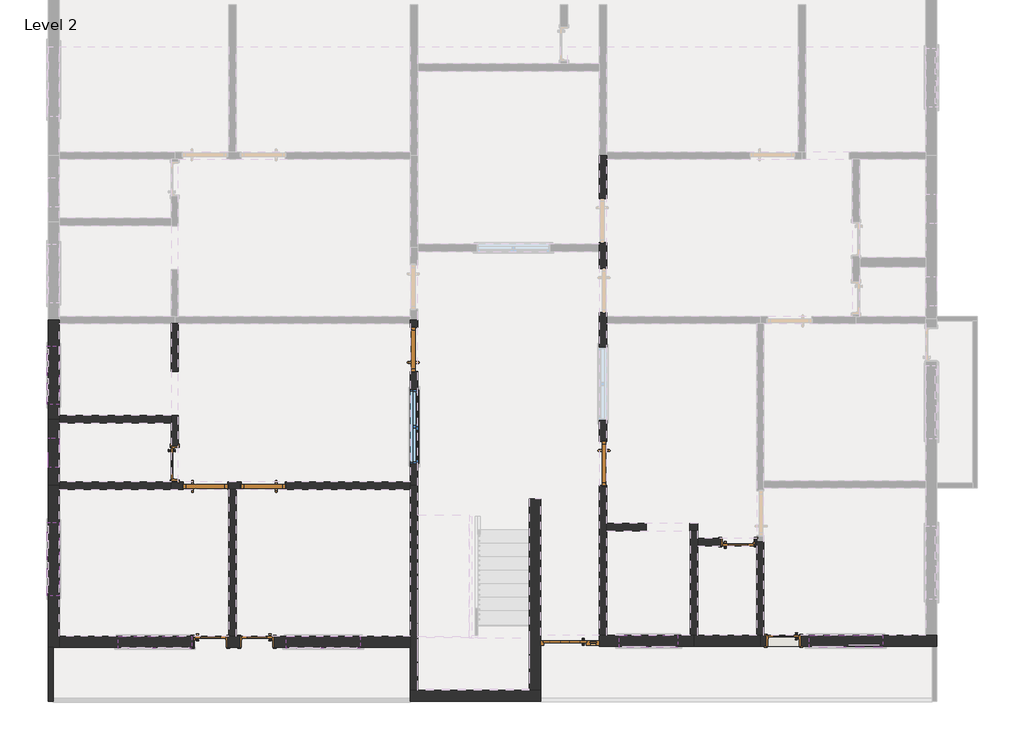
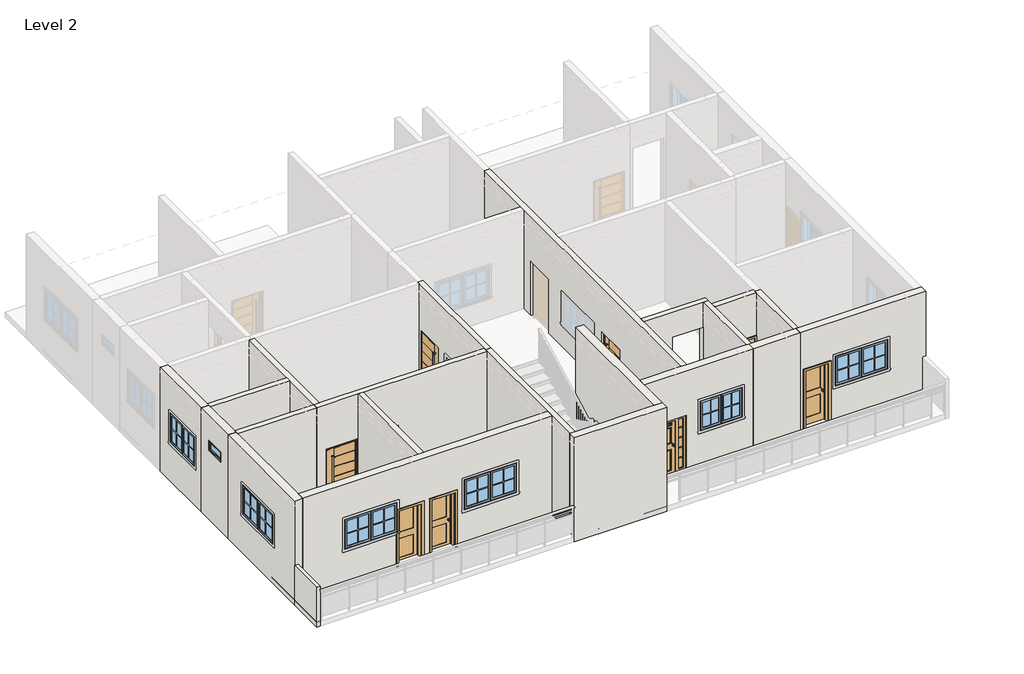
# One storey, part 1 of 5: 22 walls, 10 doors, 8 windows.
# Revit data of these elements (continued)
# Element 22 (IfcWall, "Generic - 6\"") (continued)
#   Unconnected Height = 10' - 6"
#   wall height = 10' - 6"
#   Phase Created = New Construction
#   Base Constraint = Level 2
#   Materials on its faces: "Default Wall", "BRW3", "LVW1"
# Element 23 (IfcWall, "Generic - 6\"")
#   Top Offset = 0' - 0"
#   Base Offset = 0' - 0"
#   Unconnected Height = 10' - 6"
#   wall height = 10' - 6"
#   Phase Created = New Construction
#   Base Constraint = Level 2
#   Materials on its faces: "Default Wall", "BW1", "BRW4"
# Elements 24, 27 (IfcWall, "Generic - 9\"")
#   Top Offset = 0' - 0"
#   Base Offset = 0' - 0"
#   Unconnected Height = 10' - 6"
#   wall height = 10' - 6"
#   Phase Created = New Construction
#   Base Constraint = Level 2
#   Materials on its faces: "Default Wall", "OW1", "BRW4"
# Element 25 (IfcWall, "Generic - 9\"")
#   Top Offset = 0' - 0"
#   Base Offset = 0' - 0"
#   Unconnected Height = 10' - 6"
#   wall height = 10' - 6"
#   Phase Created = New Construction
#   Base Constraint = Level 2
#   Materials on its faces: "OW1", "Default Wall", "LVW2"
# Element 26 (IfcWall, "Generic - 9\"")
#   Top Offset = 0' - 0"
#   Base Offset = 0' - 0"
#   Unconnected Height = 10' - 6"
#   wall height = 10' - 6"
#   Phase Created = New Construction
#   Base Constraint = Level 2
#   Materials on its faces: "Default Wall", "OW1"
# Element 28 (IfcWall, "Generic - 9\"")
#   Top Offset = 0' - 0"
#   Base Offset = 0' - 0"
#   Unconnected Height = 10' - 6"
#   wall height = 10' - 6"
#   Phase Created = New Construction
#   Base Constraint = Level 2
#   Materials on its faces: "Default Wall", "BW1", "OW1"
# Element 29 (IfcWall, "Generic - 9\"")
#   Top Offset = 0' - 0"
#   Base Offset = 0' - 0"
#   Unconnected Height = 10' - 6"
#   wall height = 10' - 6"
#   Phase Created = New Construction
#   Base Constraint = Level 2
#   Materials on its faces: "Default Wall", "LVW2", "OW1"
# Element 30 (IfcWall, "Generic - 9\"")
#   Top Offset = 0' - 0"
#   Base Offset = 0' - 0"
#   Unconnected Height = 10' - 6"
#   wall height = 10' - 6"
#   Phase Created = New Construction
#   Base Constraint = Level 2
#   Materials on its faces: "Default Wall", "OW1", "KW2"
# Element 31 (IfcWall, "Generic - 9\"")
#   Top Offset = 0' - 0"
#   Base Offset = 0' - 0"
#   Unconnected Height = 10' - 6"
#   wall height = 10' - 6"
#   Phase Created = New Construction
#   Base Constraint = Level 2
#   Materials on its faces: "Default Wall", "OW1", "BW1"
# Element 32 (IfcWall, "Generic - 9\"")
#   Top Offset = 0' - 0"
#   Base Offset = 0' - 0"
#   Unconnected Height = 10' - 6"
#   wall height = 10' - 6"
#   Phase Created = New Construction
#   Base Constraint = Level 2
#   Materials on its faces: "Default Wall", "OW1", "BRW3"
# Element 33 (IfcWindow, "Fixed : 2'")
#   Mark = "42"
#   Phase Created = New Construction
#   Materials on its faces: "Sash", "Glass"
# Element 34 (IfcWindow, "M_Window-Awning-Double-Horizontal : 4'")
#   Mark = "34"
#   Window Inset = 0' - 0"
#   Interior Wall Closure = 0' - 2.15551"
#   Frame Extension = 0' - 0 1/4"
#   Exterior Wall Closure = 0' - 1 1/4"
#   Interior Trim Visibility = yes
#   Exterior Trim Visibility = yes
#   Phase Created = New Construction
#   Materials on its faces: "Wood - Stained", "Glass", "Clad - White"
# Element 35 (IfcWindow, "M_Window-Awning-Double-Horizontal : 4'")
#   Mark = "35"
#   Window Inset = 0' - 0"
#   Interior Wall Closure = 0' - 2.15551"
#   Frame Extension = 0' - 0 1/4"
#   Exterior Wall Closure = 0' - 1 1/4"
#   Interior Trim Visibility = yes
#   Exterior Trim Visibility = yes
#   Phase Created = New Construction
#   Materials on its faces: "Wood - Stained", "Glass", "Clad - White"
# Element 36 (IfcWindow, "M_Window-Awning-Double-Horizontal : 5'")
#   Mark = "25"
#   Window Inset = 0' - 0"
#   Interior Wall Closure = 0' - 2 5/32"
#   Frame Extension = 0' - 0 1/4"
#   Exterior Wall Closure = 0' - 1 1/4"
#   Interior Trim Visibility = yes
#   Exterior Trim Visibility = yes
#   Phase Created = New Construction
#   Materials on its faces: "Wood - Stained", "Glass", "Clad - White"
# Element 37 (IfcWindow, "M_Window-Awning-Double-Horizontal : 5'")
#   Mark = "26"
#   Window Inset = 0' - 0"
#   Interior Wall Closure = 0' - 2 5/32"
#   Frame Extension = 0' - 0 1/4"
#   Exterior Wall Closure = 0' - 1 1/4"
#   Interior Trim Visibility = yes
#   Exterior Trim Visibility = yes
#   Phase Created = New Construction
#   Materials on its faces: "Wood - Stained", "Glass", "Clad - White"
# Element 38 (IfcWindow, "M_Window-Awning-Double-Horizontal : 5'")
#   Mark = "27"
#   Window Inset = 0' - 0"
#   Interior Wall Closure = 0' - 2 5/32"
#   Frame Extension = 0' - 0 1/4"
#   Exterior Wall Closure = 0' - 1 1/4"
#   Interior Trim Visibility = yes
#   Exterior Trim Visibility = yes
#   Phase Created = New Construction
#   Materials on its faces: "Wood - Stained", "Glass", "Clad - White"
# Element 39 (IfcWindow, "M_Window-Awning-Double-Horizontal : 5'")
#   Mark = "28"
#   Window Inset = 0' - 0"
#   Interior Wall Closure = 0' - 2 5/32"
#   Frame Extension = 0' - 0 1/4"
#   Exterior Wall Closure = 0' - 1 1/4"
#   Interior Trim Visibility = yes
#   Exterior Trim Visibility = yes
#   Phase Created = New Construction
#   Materials on its faces: "Wood - Stained", "Glass", "Clad - White"
# Element 40 (IfcWindow, "M_Window-Awning-Double-Horizontal : 5'")
#   Mark = "39"
#   Window Inset = 0' - 0"
#   Interior Wall Closure = 0' - 2.15551"
#   Frame Extension = 0' - 0 1/4"
#   Exterior Wall Closure = 0' - 1 1/4"
#   Interior Trim Visibility = yes
#   Exterior Trim Visibility = yes
#   Phase Created = New Construction
#   Materials on its faces: "Wood - Stained", "Glass", "Clad - White"
# Materials
#   "Door - Glazing": colour RGB 0 0 255, transparency 0.75
#   "Door - Panel": class "Wood", colour RGB 210 159 95, transparency 0, Cost = 0
#   "Door - Handle": colour RGB 246 240 166, transparency 0
#   "Cherry": class "Wood", colour RGB 226 177 128, transparency 0, Description = "Prunus Serotina", Cost = 0
#   "Aluminum": class "Metal", colour RGB 247 247 247, transparency 0, Description = "Aluminum 6061", Cost = 0
#   "Glass": class "Glass", colour RGB 0 128 192, transparency 0.75, Description = "Soda Lime Glass", Cost = 0
#   "Sash": class "Wood", colour RGB 224 178 126, transparency 0, Cost = 0
#   "Wood - Stained": class "Wood", colour RGB 224 178 126, transparency 0, Cost = 0
#   "Clad - White": class "Wood", colour RGB 242 242 238, transparency 0, Cost = 0
#   "Default Wall": colour RGB 128 128 128, transparency 0, Cost = 0
#   "OW1": class "Generic", colour RGB 120 120 120, transparency 0, Cost = 0
#   "BRW3": class "Generic", colour RGB 120 120 120, transparency 0, Cost = 0
#   "KW1": class "Generic", colour RGB 120 120 120, transparency 0, Cost = 0
#   "BW1": class "Generic", colour RGB 120 120 120, transparency 0, Cost = 0
#   "BRW4": class "Generic", colour RGB 120 120 120, transparency 0, Cost = 0
#   "LVW2": class "Generic", colour RGB 120 120 120, transparency 0, Cost = 0
#   "KW2": class "Generic", colour RGB 120 120 120, transparency 0, Cost = 0
#   "BRW1": class "Generic", colour RGB 120 120 120, transparency 0, Cost = 0
#   "LVW1": class "Generic", colour RGB 120 120 120, transparency 0, Cost = 0
